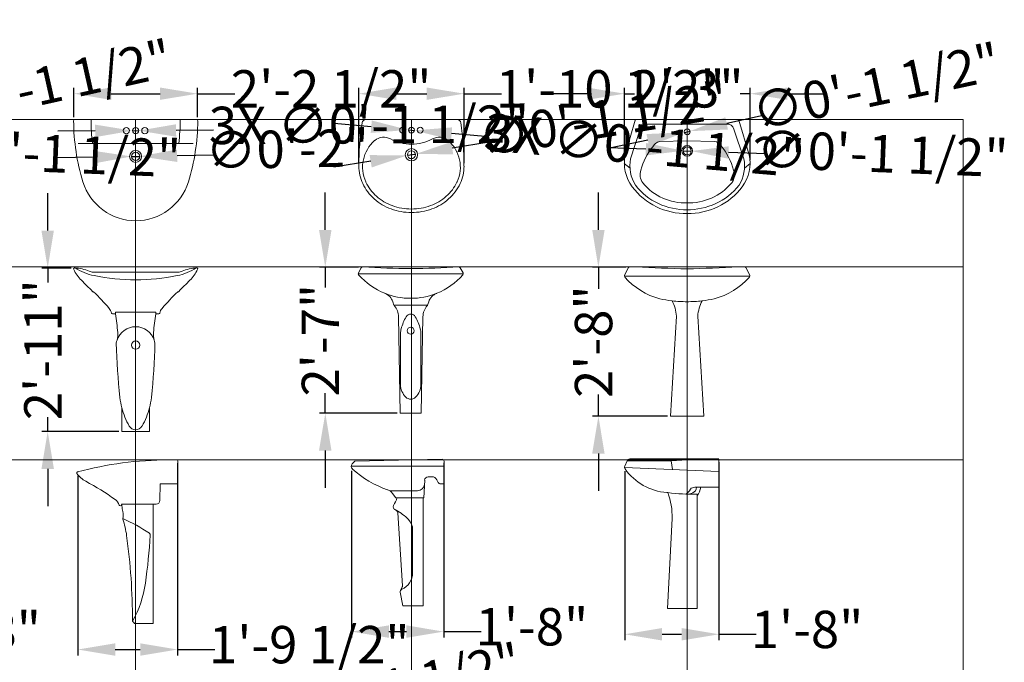
# Model space of a CAD drawing. Units: inches. Extents: x 2138 to 3265, y 2149 to 3392.
# Tile 13 of 13: x 3040 to 3251, y 3255 to 3392. Entities that reach past the tile are written whole.
import ezdxf

# ---------------------------------------------------------------- set-up
doc = ezdxf.new("R2010")
doc.units = ezdxf.units.IN
for name, color, linetype, lineweight in [('A-ANNO-DIMS', 2, 'Continuous', 18), ('A-DETL-GRID', 1, 'Continuous', 13), ('Washbasin-detail', 251, 'Continuous', 13), ('Washbasin-outline', 250, 'Continuous', 20)]:
    doc.layers.add(name, color=color, linetype=linetype, lineweight=lineweight)
doc.styles.get("Standard").update_dxf_attribs({"font": 'arial.ttf'})
doc.dimstyles.new('ISO-25', dxfattribs={"dimtxt": 8, "dimasz": 8, "dimexe": 1.25, "dimexo": 0.625, "dimtad": 0, "dimdec": 1, "dimlunit": 4, "dimtxsty": 'Standard', "dimcen": 2.5, "dimadec": 0, "dimazin": 0, "dimtfac": 1, "dimtdec": 1, "dimtmove": 0, "dimatfit": 3, "dimfxl": 1, "dimarcsym": 0})

# ---------------------------------------------------------------- blocks, each defined once
blk = doc.blocks.new('*D69')
at = {"layer": 'A-ANNO-DIMS', "color": 0, "lineweight": -2, "transparency": 16777216}
for p, q in [((2993.28, 3295.6), (2993.28, 3259.31)), ((3013.46, 3297.45), (3013.46, 3259.31)), ((3001.28, 3260.56), (3005.46, 3260.56)), ((3013.46, 3260.56), (3021.46, 3260.56))]:
    blk.add_line(p, q, dxfattribs=at)
at = {"layer": 'A-ANNO-DIMS', "color": 0, "transparency": 16777216}
for points in [[(3001.28, 3261.89), (3001.28, 3259.22), (2993.28, 3260.56)], [(3005.46, 3261.89), (3005.46, 3259.22), (3013.46, 3260.56)]]:
    blk.add_solid(points, dxfattribs=at)
at = {"layer": 'Defpoints', "color": 0, "transparency": 16777216}
for p in [(3013.46, 3298.07), (2993.28, 3296.23), (3013.46, 3260.56)]:
    blk.add_point(p, dxfattribs=at)
at = {"layer": 'A-ANNO-DIMS', "color": 0, "transparency": 16777216, "insert": (3032.34, 3260.56), "char_height": 8, "attachment_point": 5}
blk.add_mtext('1\'-8"', dxfattribs=at)
blk = doc.blocks.new('*D70')
at = {"layer": 'A-ANNO-DIMS', "color": 0, "lineweight": -2, "transparency": 16777216}
for p, q in [((3051.46, 3371.46), (3051.46, 3377.71)), ((3077.9, 3371.46), (3077.9, 3377.71)), ((3059.46, 3376.46), (3069.9, 3376.46)), ((3077.9, 3376.46), (3085.9, 3376.46))]:
    blk.add_line(p, q, dxfattribs=at)
at = {"layer": 'A-ANNO-DIMS', "color": 0, "transparency": 16777216}
for points in [[(3059.46, 3377.79), (3059.46, 3375.13), (3051.46, 3376.46)], [(3069.9, 3377.79), (3069.9, 3375.13), (3077.9, 3376.46)]]:
    blk.add_solid(points, dxfattribs=at)
at = {"layer": 'Defpoints', "color": 0, "transparency": 16777216}
for p in [(3077.9, 3376.46), (3051.46, 3370.84), (3077.9, 3370.84)]:
    blk.add_point(p, dxfattribs=at)
at = {"layer": 'A-ANNO-DIMS', "color": 0, "transparency": 16777216, "insert": (3106.55, 3376.46), "char_height": 8, "attachment_point": 5}
blk.add_mtext('2\'-2 1/2"', dxfattribs=at)
blk = doc.blocks.new('*D71')
at = {"layer": 'A-ANNO-DIMS', "color": 0, "lineweight": -2, "transparency": 16777216}
for p, q in [((3045.85, 3347.15), (3045.85, 3355.15)), ((3050.9, 3339.15), (3044.6, 3339.15)), ((3045.85, 3339.15), (3045.85, 3336.08)), ((3045.85, 3304.14), (3045.85, 3307.21)), ((3061.11, 3304.14), (3044.6, 3304.14)), ((3045.85, 3296.14), (3045.85, 3288.14))]:
    blk.add_line(p, q, dxfattribs=at)
at = {"layer": 'A-ANNO-DIMS', "color": 0, "transparency": 16777216}
for points in [[(3044.51, 3347.15), (3047.18, 3347.15), (3045.85, 3339.15)], [(3044.51, 3296.14), (3047.18, 3296.14), (3045.85, 3304.14)]]:
    blk.add_solid(points, dxfattribs=at)
at = {"layer": 'Defpoints', "color": 0, "transparency": 16777216}
for p in [(3051.53, 3339.15), (3045.85, 3304.14), (3061.73, 3304.14)]:
    blk.add_point(p, dxfattribs=at)
at = {"layer": 'A-ANNO-DIMS', "color": 0, "transparency": 16777216, "insert": (3045.85, 3321.65), "char_height": 8, "attachment_point": 5, "rotation": 90}
blk.add_mtext('2\'-11"', dxfattribs=at)
blk = doc.blocks.new('*D72')
at = {"layer": 'A-ANNO-DIMS', "color": 0, "lineweight": -2, "transparency": 16777216}
for p, q in [((3073.65, 3297.38), (3073.65, 3256.24)), ((3052.31, 3294.65), (3052.31, 3256.24)), ((3060.31, 3257.49), (3065.65, 3257.49)), ((3073.65, 3257.49), (3081.65, 3257.49))]:
    blk.add_line(p, q, dxfattribs=at)
at = {"layer": 'A-ANNO-DIMS', "color": 0, "transparency": 16777216}
for points in [[(3060.31, 3258.82), (3060.31, 3256.15), (3052.31, 3257.49)], [(3065.65, 3258.82), (3065.65, 3256.15), (3073.65, 3257.49)]]:
    blk.add_solid(points, dxfattribs=at)
at = {"layer": 'Defpoints', "color": 0, "transparency": 16777216}
for p in [(3073.65, 3298.01), (3052.31, 3295.28), (3073.65, 3257.49)]:
    blk.add_point(p, dxfattribs=at)
at = {"layer": 'A-ANNO-DIMS', "color": 0, "transparency": 16777216, "insert": (3101.86, 3257.49), "char_height": 8, "attachment_point": 5}
blk.add_mtext('1\'-9 1/2"', dxfattribs=at)
blk = doc.blocks.new('*D73')
at = {"layer": 'A-ANNO-DIMS', "color": 0, "lineweight": -2, "transparency": 16777216}
for p, q in [((3112.48, 3361.59), (3112.48, 3377.71)), ((3135, 3361.59), (3135, 3377.71)), ((3120.48, 3376.46), (3127, 3376.46)), ((3135, 3376.46), (3143, 3376.46))]:
    blk.add_line(p, q, dxfattribs=at)
at = {"layer": 'A-ANNO-DIMS', "color": 0, "transparency": 16777216}
for points in [[(3120.48, 3377.79), (3120.48, 3375.13), (3112.48, 3376.46)], [(3127, 3377.79), (3127, 3375.13), (3135, 3376.46)]]:
    blk.add_solid(points, dxfattribs=at)
at = {"layer": 'Defpoints', "color": 0, "transparency": 16777216}
for p in [(3135, 3376.46), (3112.48, 3360.96), (3135, 3360.96)]:
    blk.add_point(p, dxfattribs=at)
at = {"layer": 'A-ANNO-DIMS', "color": 0, "transparency": 16777216, "insert": (3166.31, 3376.46), "char_height": 8, "attachment_point": 5}
blk.add_mtext('1\'-10 1/2"', dxfattribs=at)
blk = doc.blocks.new('*D74')
at = {"layer": 'A-ANNO-DIMS', "color": 0, "lineweight": -2, "transparency": 16777216}
for p, q in [((3105.29, 3347.3), (3105.29, 3355.3)), ((3112.41, 3339.3), (3104.04, 3339.3)), ((3105.29, 3339.3), (3105.29, 3335.01)), ((3105.29, 3308.08), (3105.29, 3312.36)), ((3120.71, 3308.08), (3104.04, 3308.08)), ((3105.29, 3300.08), (3105.29, 3292.08))]:
    blk.add_line(p, q, dxfattribs=at)
at = {"layer": 'A-ANNO-DIMS', "color": 0, "transparency": 16777216}
for points in [[(3103.95, 3347.3), (3106.62, 3347.3), (3105.29, 3339.3)], [(3103.95, 3300.08), (3106.62, 3300.08), (3105.29, 3308.08)]]:
    blk.add_solid(points, dxfattribs=at)
at = {"layer": 'Defpoints', "color": 0, "transparency": 16777216}
for p in [(3113.03, 3339.3), (3105.29, 3308.08), (3121.34, 3308.08)]:
    blk.add_point(p, dxfattribs=at)
at = {"layer": 'A-ANNO-DIMS', "color": 0, "transparency": 16777216, "insert": (3105.29, 3323.69), "char_height": 8, "attachment_point": 5, "rotation": 90}
blk.add_mtext('2\'-7"', dxfattribs=at)
blk = doc.blocks.new('*D75')
at = {"layer": 'A-ANNO-DIMS', "color": 0, "lineweight": -2, "transparency": 16777216}
for p, q in [((3110.91, 3295.76), (3110.91, 3260.07)), ((3130.66, 3297.42), (3130.66, 3260.07)), ((3118.91, 3261.32), (3122.66, 3261.32)), ((3130.66, 3261.32), (3138.66, 3261.32))]:
    blk.add_line(p, q, dxfattribs=at)
at = {"layer": 'A-ANNO-DIMS', "color": 0, "transparency": 16777216}
for points in [[(3118.91, 3262.66), (3118.91, 3259.99), (3110.91, 3261.32)], [(3122.66, 3262.66), (3122.66, 3259.99), (3130.66, 3261.32)]]:
    blk.add_solid(points, dxfattribs=at)
at = {"layer": 'Defpoints', "color": 0, "transparency": 16777216}
for p in [(3130.66, 3298.04), (3110.91, 3296.39), (3130.66, 3261.32)]:
    blk.add_point(p, dxfattribs=at)
at = {"layer": 'A-ANNO-DIMS', "color": 0, "transparency": 16777216, "insert": (3149.54, 3261.32), "char_height": 8, "attachment_point": 5}
blk.add_mtext('1\'-8"', dxfattribs=at)
blk = doc.blocks.new('*D76')
at = {"layer": 'A-ANNO-DIMS', "color": 0, "lineweight": -2, "transparency": 16777216}
for p, q in [((3169.33, 3362.21), (3169.33, 3377.71)), ((3196.26, 3362.21), (3196.26, 3377.71)), ((3161.33, 3376.46), (3153.33, 3376.46)), ((3169.33, 3376.46), (3171.47, 3376.46)), ((3196.26, 3376.46), (3194.12, 3376.46)), ((3204.26, 3376.46), (3212.26, 3376.46))]:
    blk.add_line(p, q, dxfattribs=at)
at = {"layer": 'A-ANNO-DIMS', "color": 0, "transparency": 16777216}
for points in [[(3161.33, 3377.79), (3161.33, 3375.13), (3169.33, 3376.46)], [(3204.26, 3377.79), (3204.26, 3375.13), (3196.26, 3376.46)]]:
    blk.add_solid(points, dxfattribs=at)
at = {"layer": 'Defpoints', "color": 0, "transparency": 16777216}
for p in [(3196.26, 3376.46), (3169.33, 3361.58), (3196.26, 3361.58)]:
    blk.add_point(p, dxfattribs=at)
at = {"layer": 'A-ANNO-DIMS', "color": 0, "transparency": 16777216, "insert": (3182.8, 3376.46), "char_height": 8, "attachment_point": 5}
blk.add_mtext('2\'-3"', dxfattribs=at)
blk = doc.blocks.new('*D77')
at = {"layer": 'A-ANNO-DIMS', "color": 0, "lineweight": -2, "transparency": 16777216}
for p, q in [((3163.77, 3347.31), (3163.77, 3355.31)), ((3169.65, 3339.31), (3162.52, 3339.31)), ((3163.77, 3339.31), (3163.77, 3334.7)), ((3163.77, 3307.44), (3163.77, 3312.05)), ((3178.59, 3307.44), (3162.52, 3307.44)), ((3163.77, 3299.44), (3163.77, 3291.44))]:
    blk.add_line(p, q, dxfattribs=at)
at = {"layer": 'A-ANNO-DIMS', "color": 0, "transparency": 16777216}
for points in [[(3162.44, 3347.31), (3165.1, 3347.31), (3163.77, 3339.31)], [(3162.44, 3299.44), (3165.1, 3299.44), (3163.77, 3307.44)]]:
    blk.add_solid(points, dxfattribs=at)
at = {"layer": 'Defpoints', "color": 0, "transparency": 16777216}
for p in [(3170.27, 3339.31), (3163.77, 3307.44), (3179.21, 3307.44)]:
    blk.add_point(p, dxfattribs=at)
at = {"layer": 'A-ANNO-DIMS', "color": 0, "transparency": 16777216, "insert": (3163.77, 3323.38), "char_height": 8, "attachment_point": 5, "rotation": 90}
blk.add_mtext('2\'-8"', dxfattribs=at)
blk = doc.blocks.new('*D78')
at = {"layer": 'A-ANNO-DIMS', "color": 0, "lineweight": -2, "transparency": 16777216}
for p, q in [((3189.57, 3297.61), (3189.57, 3259.5)), ((3169.41, 3295.65), (3169.41, 3259.5)), ((3177.41, 3260.75), (3181.57, 3260.75)), ((3189.57, 3260.75), (3197.57, 3260.75))]:
    blk.add_line(p, q, dxfattribs=at)
at = {"layer": 'A-ANNO-DIMS', "color": 0, "transparency": 16777216}
for points in [[(3177.41, 3262.09), (3177.41, 3259.42), (3169.41, 3260.75)], [(3181.57, 3262.09), (3181.57, 3259.42), (3189.57, 3260.75)]]:
    blk.add_solid(points, dxfattribs=at)
at = {"layer": 'Defpoints', "color": 0, "transparency": 16777216}
for p in [(3189.57, 3298.23), (3169.41, 3296.27), (3189.57, 3260.75)]:
    blk.add_point(p, dxfattribs=at)
at = {"layer": 'A-ANNO-DIMS', "color": 0, "transparency": 16777216, "insert": (3208.45, 3260.75), "char_height": 8, "attachment_point": 5}
blk.add_mtext('1\'-8"', dxfattribs=at)
blk = doc.blocks.new('*D113')
at = {"layer": 'A-ANNO-DIMS', "color": 0, "lineweight": -2, "transparency": 16777216}
for p, q in [((3021.86, 3371.95), (3014.05, 3370.2)), ((3005.01, 3368.17), (3006.24, 3368.45)), ((2997.21, 3366.42), (2989.4, 3364.68))]:
    blk.add_line(p, q, dxfattribs=at)
at = {"layer": 'A-ANNO-DIMS', "color": 0, "transparency": 16777216}
for points in [[(3013.76, 3371.5), (3014.34, 3368.9), (3006.24, 3368.45)], [(2996.92, 3367.73), (2997.5, 3365.12), (3005.01, 3368.17)]]:
    blk.add_solid(points, dxfattribs=at)
at = {"layer": 'Defpoints', "color": 0, "transparency": 16777216}
for p in [(3005.01, 3368.17), (3006.24, 3368.45)]:
    blk.add_point(p, dxfattribs=at)
at = {"layer": 'A-ANNO-DIMS', "color": 0, "transparency": 16777216, "insert": (3046.18, 3377.39), "char_height": 8, "attachment_point": 5, "rotation": 12.6253}
blk.add_mtext('∅0\'-1 1/2"', dxfattribs=at)
blk = doc.blocks.new('*D114')
at = {"layer": 'A-ANNO-DIMS', "color": 0, "lineweight": -2, "transparency": 16777216}
for p, q in [((2996.77, 3364.56), (2988.77, 3364.88)), ((3004.76, 3364.25), (3006.49, 3364.18)), ((3022.48, 3363.55), (3014.49, 3363.87))]:
    blk.add_line(p, q, dxfattribs=at)
at = {"layer": 'A-ANNO-DIMS', "color": 0, "transparency": 16777216}
for points in [[(2996.82, 3365.9), (2996.72, 3363.23), (3004.76, 3364.25)], [(3014.54, 3365.2), (3014.44, 3362.54), (3006.49, 3364.18)]]:
    blk.add_solid(points, dxfattribs=at)
at = {"layer": 'Defpoints', "color": 0, "transparency": 16777216}
for p in [(3004.76, 3364.25), (3006.49, 3364.18)]:
    blk.add_point(p, dxfattribs=at)
at = {"layer": 'A-ANNO-DIMS', "color": 0, "transparency": 16777216, "insert": (3047.39, 3362.58), "char_height": 8, "attachment_point": 5, "rotation": 357.7522}
blk.add_mtext('∅0\'-1 1/2"', dxfattribs=at)
blk = doc.blocks.new('*D115')
at = {"layer": 'A-ANNO-DIMS', "color": 0, "lineweight": -2, "transparency": 16777216}
for p, q in [((3056.01, 3368.51), (3048.01, 3368.47)), ((3064.01, 3368.54), (3065.35, 3368.55)), ((3081.35, 3368.62), (3073.35, 3368.59))]:
    blk.add_line(p, q, dxfattribs=at)
at = {"layer": 'A-ANNO-DIMS', "color": 0, "transparency": 16777216}
for points in [[(3056.01, 3369.84), (3056.02, 3367.17), (3064.01, 3368.54)], [(3073.35, 3369.92), (3073.36, 3367.25), (3065.35, 3368.55)]]:
    blk.add_solid(points, dxfattribs=at)
at = {"layer": 'Defpoints', "color": 0, "transparency": 16777216}
for p in [(3064.01, 3368.54), (3065.35, 3368.55)]:
    blk.add_point(p, dxfattribs=at)
at = {"layer": 'A-ANNO-DIMS', "color": 0, "transparency": 16777216, "insert": (3114.66, 3368.78), "char_height": 8, "attachment_point": 5, "rotation": 0.2663}
blk.add_mtext('3X ∅0\'-1 1/2"', dxfattribs=at)
blk = doc.blocks.new('*D116')
at = {"layer": 'A-ANNO-DIMS', "color": 0, "lineweight": -2, "transparency": 16777216}
for p, q in [((3055.8, 3362.89), (3047.8, 3362.75)), ((3063.8, 3363.02), (3065.57, 3363.05)), ((3081.57, 3363.32), (3073.57, 3363.18))]:
    blk.add_line(p, q, dxfattribs=at)
at = {"layer": 'A-ANNO-DIMS', "color": 0, "transparency": 16777216}
for points in [[(3055.78, 3364.22), (3055.82, 3361.55), (3063.8, 3363.02)], [(3073.55, 3364.52), (3073.59, 3361.85), (3065.57, 3363.05)]]:
    blk.add_solid(points, dxfattribs=at)
at = {"layer": 'Defpoints', "color": 0, "transparency": 16777216}
for p in [(3063.8, 3363.02), (3065.57, 3363.05)]:
    blk.add_point(p, dxfattribs=at)
at = {"layer": 'A-ANNO-DIMS', "color": 0, "transparency": 16777216, "insert": (3097.17, 3363.58), "char_height": 8, "attachment_point": 5, "rotation": 0.9632}
blk.add_mtext('∅0\'-2"', dxfattribs=at)
blk = doc.blocks.new('*D117')
at = {"layer": 'A-ANNO-DIMS', "color": 0, "lineweight": -2, "transparency": 16777216}
for p, q in [((3115.13, 3369.4), (3107.16, 3370.08)), ((3123.1, 3368.71), (3124.37, 3368.6)), ((3140.32, 3367.24), (3132.34, 3367.92))]:
    blk.add_line(p, q, dxfattribs=at)
at = {"layer": 'A-ANNO-DIMS', "color": 0, "transparency": 16777216}
for points in [[(3115.25, 3370.72), (3115.02, 3368.07), (3123.1, 3368.71)], [(3132.46, 3369.25), (3132.23, 3366.59), (3124.37, 3368.6)]]:
    blk.add_solid(points, dxfattribs=at)
at = {"layer": 'Defpoints', "color": 0, "transparency": 16777216}
for p in [(3123.1, 3368.71), (3124.37, 3368.6)]:
    blk.add_point(p, dxfattribs=at)
at = {"layer": 'A-ANNO-DIMS', "color": 0, "transparency": 16777216, "insert": (3173.5, 3364.39), "char_height": 8, "attachment_point": 5, "rotation": 355.1005}
blk.add_mtext('3X ∅0\'-1 1/2"', dxfattribs=at)
blk = doc.blocks.new('*D118')
at = {"layer": 'A-ANNO-DIMS', "color": 0, "lineweight": -2, "transparency": 16777216}
for p, q in [((3140.37, 3366.1), (3132.47, 3364.82)), ((3122.9, 3363.27), (3124.57, 3363.54)), ((3115.01, 3361.99), (3107.11, 3360.71))]:
    blk.add_line(p, q, dxfattribs=at)
at = {"layer": 'A-ANNO-DIMS', "color": 0, "transparency": 16777216}
for points in [[(3132.26, 3366.13), (3132.68, 3363.5), (3124.57, 3363.54)], [(3114.79, 3363.31), (3115.22, 3360.67), (3122.9, 3363.27)]]:
    blk.add_solid(points, dxfattribs=at)
at = {"layer": 'Defpoints', "color": 0, "transparency": 16777216}
for p in [(3122.9, 3363.27), (3124.57, 3363.54)]:
    blk.add_point(p, dxfattribs=at)
at = {"layer": 'A-ANNO-DIMS', "color": 0, "transparency": 16777216, "insert": (3164.98, 3370.08), "char_height": 8, "attachment_point": 5, "rotation": 9.1943}
blk.add_mtext('∅0\'-1 1/2"', dxfattribs=at)
blk = doc.blocks.new('*D119')
at = {"layer": 'A-ANNO-DIMS', "color": 0, "lineweight": -2, "transparency": 16777216}
for p, q in [((3199.06, 3371.76), (3191.24, 3370.1)), ((3182.18, 3368.18), (3183.41, 3368.44)), ((3174.35, 3366.52), (3166.53, 3364.86))]:
    blk.add_line(p, q, dxfattribs=at)
at = {"layer": 'A-ANNO-DIMS', "color": 0, "transparency": 16777216}
for points in [[(3190.96, 3371.41), (3191.51, 3368.8), (3183.41, 3368.44)], [(3174.07, 3367.82), (3174.63, 3365.22), (3182.18, 3368.18)]]:
    blk.add_solid(points, dxfattribs=at)
at = {"layer": 'Defpoints', "color": 0, "transparency": 16777216}
for p in [(3182.18, 3368.18), (3183.41, 3368.44)]:
    blk.add_point(p, dxfattribs=at)
at = {"layer": 'A-ANNO-DIMS', "color": 0, "transparency": 16777216, "insert": (3223.45, 3376.94), "char_height": 8, "attachment_point": 5, "rotation": 11.979}
blk.add_mtext('∅0\'-1 1/2"', dxfattribs=at)
blk = doc.blocks.new('*D120')
at = {"layer": 'A-ANNO-DIMS', "color": 0, "lineweight": -2, "transparency": 16777216}
for p, q in [((3173.93, 3364.56), (3165.94, 3364.87)), ((3181.93, 3364.25), (3183.66, 3364.18)), ((3199.65, 3363.56), (3191.65, 3363.87))]:
    blk.add_line(p, q, dxfattribs=at)
at = {"layer": 'A-ANNO-DIMS', "color": 0, "transparency": 16777216}
for points in [[(3173.99, 3365.89), (3173.88, 3363.23), (3181.93, 3364.25)], [(3191.7, 3365.2), (3191.6, 3362.54), (3183.66, 3364.18)]]:
    blk.add_solid(points, dxfattribs=at)
at = {"layer": 'Defpoints', "color": 0, "transparency": 16777216}
for p in [(3181.93, 3364.25), (3183.66, 3364.18)]:
    blk.add_point(p, dxfattribs=at)
at = {"layer": 'A-ANNO-DIMS', "color": 0, "transparency": 16777216, "insert": (3224.56, 3362.59), "char_height": 8, "attachment_point": 5, "rotation": 357.7634}
blk.add_mtext('∅0\'-1 1/2"', dxfattribs=at)
blk = doc.blocks.new('*D125')
at = {"layer": 'A-ANNO-DIMS', "color": 0, "lineweight": -2, "transparency": 16777216}
for p, q in [((3080.99, 3240.1), (3073.17, 3238.45)), ((3064.03, 3236.52), (3065.34, 3236.8)), ((3056.2, 3234.87), (3048.37, 3233.21))]:
    blk.add_line(p, q, dxfattribs=at)
at = {"layer": 'A-ANNO-DIMS', "color": 0, "transparency": 16777216}
for points in [[(3072.89, 3239.75), (3073.44, 3237.14), (3065.34, 3236.8)], [(3055.93, 3236.17), (3056.48, 3233.56), (3064.03, 3236.52)]]:
    blk.add_solid(points, dxfattribs=at)
at = {"layer": 'Defpoints', "color": 0, "transparency": 16777216}
for p in [(3064.03, 3236.52), (3065.34, 3236.8)]:
    blk.add_point(p, dxfattribs=at)
at = {"layer": 'A-ANNO-DIMS', "color": 0, "transparency": 16777216, "insert": (3113.58, 3246.98), "char_height": 8, "attachment_point": 5, "rotation": 11.9181}
blk.add_mtext('3X ∅0\'-1 1/2"', dxfattribs=at)

msp = doc.modelspace()

# ---------------------------------------------------------------- linework, layer by layer
at = {"layer": 'A-DETL-GRID'}
for p, q in [((2828.46, 3370.91), (3241.85, 3370.91)), ((3064.68, 3239.02), (3064.68, 3370.91)), ((3123.74, 3239.02), (3123.74, 3370.91)), ((3182.79, 3239.02), (3182.79, 3370.91)), ((3241.85, 3239.02), (3241.85, 3370.91)), ((2828.46, 3339.41), (3241.85, 3339.41)), ((2828.46, 3298.07), (3241.85, 3298.07))]:
    msp.add_line(p, q, dxfattribs=at)
at = {"layer": 'Washbasin-detail'}
for p, q in [((3170.54, 3360.51), (3169.32, 3361.5)), ((3195.05, 3360.51), (3196.27, 3361.5)), ((3064.68, 3338.27), (3055.63, 3338.27)), ((3064.68, 3338.27), (3073.74, 3338.27)), ((3112.33, 3337.91), (3123.59, 3337.91)), ((3113.31, 3339.41), (3123.59, 3339.41)), ((3133.87, 3339.41), (3123.59, 3339.41)), ((3134.84, 3337.91), (3123.59, 3337.91)), ((3120.03, 3331.16), (3123.59, 3331.16)), ((3127.15, 3331.16), (3123.59, 3331.16)), ((3121.4, 3325.14), (3121.4, 3314.2)), ((3125.77, 3325.14), (3125.77, 3314.2)), ((3061.73, 3304.14), (3061.73, 3309.2)), ((3067.64, 3304.14), (3067.64, 3309.2)), ((3064.68, 3304.14), (3061.73, 3304.14)), ((3064.68, 3304.14), (3067.64, 3304.14)), ((3110.84, 3296.71), (3130.72, 3296.71)), ((3120.63, 3289.95), (3126.24, 3289.95)), ((3061.8, 3288.63), (3068.41, 3288.63)), ((3061.8, 3288.63), (3062.61, 3288.63)), ((3123.99, 3283.2), (3123.99, 3273.86))]:
    msp.add_line(p, q, dxfattribs=at)
for points in [[(3182.79, 3369.92), (3174.29, 3369.92, 0.390337), (3172.71, 3368.9), (3170.66, 3362.55, 0.183446), (3171.69, 3356.85, 0.232242), (3182.79, 3351.62, 0.646667)], [(3182.79, 3369.92), (3191.19, 3369.92, -0.390337), (3192.76, 3368.9), (3194.94, 3362.55, -0.183446), (3193.9, 3356.85, -0.230237), (3182.68, 3351.62, -0.646667)], [(3113.96, 3357.61, 0.00234), (3113.99, 3357.54, 0.102555), (3116.27, 3354.5, 0.093464), (3119.63, 3352.5, 0.087915), (3123.74, 3351.77, 0.087915)], [(3133.51, 3357.61, -0.00234), (3133.48, 3357.54, -0.102555), (3131.2, 3354.5, -0.093464), (3127.85, 3352.5, -0.087915), (3123.74, 3351.77, -0.087915)], [(3182.79, 3338.98, -0.010807), (3171.81, 3339.41, -32.766404)], [(3182.74, 3338.98, 0.010807), (3193.73, 3339.41, 32.766404)], [(3184.76, 3292.21, -0.342017), (3183.97, 3291.03, -0.117748), (3182.71, 3290.71, 189.338615)], [(3185.67, 3292.21, -0.172288), (3184.92, 3290.45, 0.079687)]]:
    msp.add_lwpolyline(points, format="xyb", dxfattribs=at)
for points in [[(3182.79, 3337.41), (3169.37, 3337.41)], [(3182.74, 3337.41), (3196.17, 3337.41)], [(3169.92, 3297.88), (3179.37, 3297.88), (3186.22, 3298.27)], [(3179.37, 3297.88), (3179.64, 3296)], [(3169.37, 3296.42), (3189.57, 3295.59)]]:
    msp.add_lwpolyline(points, dxfattribs=at)
for centre, radius in [((3062.71, 3368.55), 0.669), ((3064.68, 3368.55), 0.669), ((3066.65, 3368.55), 0.669), ((3121.86, 3368.66), 0.638), ((3125.61, 3368.66), 0.638), ((3182.79, 3368.31), 0.63), ((3182.79, 3364.22), 1.14), ((3182.79, 3364.22), 0.866), ((3064.68, 3363.04), 1.28), ((3064.68, 3363.04), 0.886), ((3123.74, 3363.4), 1.31), ((3123.59, 3325.72), 0.751), ((3064.68, 3322.64), 0.886)]:
    msp.add_circle(centre, radius, dxfattribs=at)
for centre, radius, start, end in [((3096.66, 3370.9), 41.53, 179.9856, 187.0649), ((3032.7, 3370.9), 41.53, 352.9351, 0.0144), ((3123.74, 3368.66), 0.638, 90, 270), ((3123.74, 3368.66), 0.638, 270, 90), ((3117.83, 3364.15), 3, 61.4965, 130.9137), ((3129.65, 3364.15), 3, 49.0863, 118.5035), ((3120.78, 3360.75), 7.51, 130.9137, 204.754), ((3123.74, 3375.04), 9.38, 241.4965, 270), ((3123.74, 3375.04), 9.38, 270, 298.5035), ((3126.7, 3360.75), 7.51, 335.246, 49.0863), ((3123.74, 3363.4), 0.844, 90, 270), ((3123.74, 3363.4), 0.844, 270, 90), ((3050.96, 3329.36), 9.84, 67.5001, 85.9904), ((3055.63, 3340.64), 2.36, 247.5001, 270), ((3073.74, 3340.64), 2.36, 270, 292.4999), ((3078.41, 3329.36), 9.84, 94.0096, 112.4999), ((3123.59, 3328.16), 1.13, 90, 150.274), ((3123.59, 3328.16), 1.13, 29.726, 90), ((3132.39, 3323.13), 11.26, 150.274, 164.5121), ((3114.79, 3323.13), 11.26, 15.4879, 29.726), ((3125.15, 3325.14), 3.75, 164.5121, 180), ((3122.02, 3325.14), 3.75, 0, 15.4879), ((3125.15, 3314.2), 3.75, 180, 225.9297), ((3122.02, 3314.2), 3.75, 314.0703, 0), ((3123.59, 3312.58), 1.5, 225.9297, 270), ((3123.59, 3312.58), 1.5, 270, 314.0703), ((3115.12, 3277.39), 11.26, 44.6785, 61.8252), ((3049.56, 3256.55), 31.5, 55.0237, 66.9079), ((3120.99, 3283.2), 3, 0, 44.6785), ((2934.23, 3290.44), 133.86, 351.9594, 356.3821), ((3067.43, 3282.01), 0.394, 356.3821, 61.0641), ((3120.24, 3273.86), 3.75, 292.458, 0), ((3043.38, 3275.02), 23.62, 330.9388, 351.9594)]:
    msp.add_arc(centre, radius, start, end, dxfattribs=at)
at = {"layer": 'Washbasin-outline'}
for p, q in [((3051.63, 3370.91), (3077.73, 3370.91)), ((3113.93, 3370.91), (3123.74, 3370.91)), ((3133.55, 3370.91), (3123.74, 3370.91)), ((3052.35, 3365.79), (3064.68, 3365.79)), ((3077.02, 3365.79), (3064.68, 3365.79)), ((3112.97, 3339.21), (3112.37, 3338.09)), ((3134.2, 3339.21), (3134.8, 3338.09)), ((3169.36, 3337.59), (3170.22, 3339.24)), ((3170.51, 3339.41), (3182.79, 3339.41)), ((3195.02, 3339.41), (3182.74, 3339.41)), ((3196.18, 3337.59), (3195.31, 3339.24)), ((3055.68, 3334.06), (3055.59, 3334.06)), ((3073.69, 3334.06), (3073.78, 3334.06)), ((3120, 3331.21), (3119.75, 3331.94)), ((3127.15, 3331.16), (3127.43, 3331.94)), ((3060.36, 3329.34), (3059.74, 3329.34)), ((3060.36, 3329.34), (3060.36, 3329.73)), ((3064.68, 3329.73), (3060.36, 3329.73)), ((3064.68, 3329.73), (3069.01, 3329.73)), ((3069.01, 3329.34), (3069.01, 3329.73)), ((3069.62, 3329.34), (3069.01, 3329.34)), ((3121.34, 3308.08), (3120.98, 3328.71)), ((3125.84, 3308.08), (3126.2, 3328.71)), ((3121.34, 3308.08), (3125.84, 3308.08)), ((3071.67, 3298.07), (3073.49, 3298.07)), ((3073.72, 3297.84), (3073.72, 3292.96)), ((3111.59, 3297.83), (3111.03, 3297.21)), ((3111.59, 3297.83), (3130.34, 3298.21)), ((3130.72, 3297.83), (3130.72, 3293.1)), ((3169.42, 3296.74), (3169.91, 3297.89)), ((3170.49, 3298.27), (3189.57, 3298.27)), ((3126.41, 3289.95), (3126.57, 3293.73)), ((3127.32, 3294.45), (3128.15, 3294.45)), ((3129.44, 3293.26), (3129.16, 3293.83)), ((3069.88, 3289.4), (3069.92, 3292.96)), ((3069.92, 3292.96), (3073.72, 3292.96)), ((3119.09, 3291.45), (3125.03, 3291.45)), ((3129.95, 3292.95), (3130.57, 3292.95)), ((3120.4, 3289.95), (3119.7, 3290.89)), ((3120.4, 3289.95), (3120.63, 3289.95)), ((3126.24, 3289.95), (3126.24, 3266.87)), ((3126.24, 3289.95), (3126.41, 3289.95)), ((3184.92, 3290.45), (3184.92, 3290.71)), ((3184.92, 3266.3), (3184.92, 3290.45)), ((3061.65, 3288.42), (3061.69, 3288.54)), ((3061.72, 3288.63), (3061.72, 3288.23)), ((3061.72, 3288.63), (3061.8, 3288.63)), ((3068.41, 3288.63), (3068.41, 3263.04)), ((3068.41, 3288.63), (3069.09, 3288.63)), ((3120.83, 3286.71), (3121.81, 3271.09)), ((3121.38, 3270.12), (3121.78, 3270.92)), ((3121.34, 3269.77), (3121.89, 3266.87)), ((3121.89, 3266.87), (3126.24, 3266.87)), ((3064.47, 3263.04), (3068.41, 3263.04))]:
    msp.add_line(p, q, dxfattribs=at)
for points in [[(3051.4, 3370.67, 0.07343), (3053.39, 3357.6, 0.07343)], [(3182.79, 3370.91), (3171.81, 3370.91, 0.349334), (3171.62, 3370.76), (3169.5, 3363.39, 0.210862), (3171.01, 3356.53, 0.238221), (3182.75, 3350.79, -0.006376)], [(3182.79, 3370.91), (3193.67, 3370.91, -0.349334), (3193.86, 3370.76), (3196.09, 3363.39, -0.210862), (3194.58, 3356.53, -0.236938), (3182.76, 3350.79, 0.006376)], [(3182.79, 3366.34), (3176.83, 3366.24, 0.204561), (3175.43, 3365.12, 0.107345), (3172.89, 3360.11, 0.24654), (3173.27, 3357.37, 0.234802), (3182.83, 3353.11, 0.791678)], [(3182.68, 3366.34), (3188.64, 3366.24, -0.218686), (3190.04, 3365.32, -0.103144), (3192.71, 3360.11, -0.24654), (3192.33, 3357.37, -0.232404), (3182.64, 3353.11, -0.791678)], [(3112.48, 3360.96, 0.11006), (3113.31, 3357.22, 0.102555), (3115.78, 3353.93, 0.093464), (3119.37, 3351.8, 0.087915), (3123.74, 3351.02, 0.087915)], [(3135, 3360.96, -0.11006), (3134.16, 3357.22, -0.102555), (3131.7, 3353.93, -0.093464), (3128.11, 3351.8, -0.087915), (3123.74, 3351.02, -0.087915)], [(3053.39, 3357.6, 0.329453), (3064.68, 3349.26, 0.329453), (3075.97, 3357.6, 0.329453)], [(3182.79, 3307.44), (3179.21, 3307.44), (3180.5, 3328.86, 0.094609), (3179.54, 3332.13, -1.525098)], [(3182.74, 3307.44), (3186.32, 3307.44), (3185.03, 3328.86, -0.094609), (3186, 3332.13, 1.525098)], [(3189.57, 3298.23), (3189.57, 3292.21), (3185.67, 3292.21, 0.240306)], [(3185.67, 3292.21), (3184.41, 3292.21, 0.240306), (3183.46, 3291.81, -0.219906), (3182.32, 3290.75, 6.2607)], [(3184.92, 3266.3), (3178.54, 3266.3), (3179.55, 3285.55, 0.103398), (3178.61, 3291.08, 5.161723)]]:
    msp.add_lwpolyline(points, format="xyb", dxfattribs=at)
for centre, radius, start, end in [((3051.63, 3370.67), 0.236, 90, 180.2872), ((3032.7, 3370.9), 45.28, 342.9141, 359.7128), ((3077.73, 3370.67), 0.236, 359.7128, 90), ((3174.46, 3360.96), 61.98, 171.3647, 180), ((3113.93, 3370.16), 0.751, 90, 171.3647), ((3133.55, 3370.16), 0.751, 4.4701, 90), ((3073.01, 3360.96), 61.98, 360, 8.6353), ((3051.63, 3338.94), 0.236, 85.9904, 205.7315), ((3059.22, 3342.6), 8.66, 205.7315, 224.658), ((3058.12, 3349.09), 11.81, 237.0913, 258.5261), ((3071.24, 3349.09), 11.81, 281.4739, 302.9087), ((3070.14, 3342.6), 8.66, 315.342, 334.2685), ((3077.73, 3338.94), 0.236, 334.2685, 94.0096), ((3112.7, 3337.91), 0.375, 151.9275, 221.7089), ((3123.59, 3347.61), 14.95, 221.7089, 248.1891), ((3113.31, 3339.04), 0.375, 90, 151.9275), ((3123.59, 3480.09), 141.05, 265.8197, 274.1803), ((3123.59, 3347.61), 14.95, 291.8109, 318.2911), ((3133.87, 3339.04), 0.375, 28.0725, 90), ((3134.47, 3337.91), 0.375, 318.2911, 28.0725), ((3169.65, 3337.44), 0.325, 152.4267, 221.363), ((3170.51, 3339.09), 0.325, 90, 152.4267), ((3195.02, 3339.09), 0.325, 27.5733, 90), ((3195.89, 3337.44), 0.325, 318.637, 27.5733), ((3012.28, 3293.8), 59.06, 43.0851, 46.3304), ((3064.68, 3381.41), 44.79, 258.5261, 270), ((3064.68, 3381.41), 44.79, 270, 281.4739), ((3117.08, 3293.8), 59.06, 133.6696, 136.9149), ((3180.87, 3347.32), 15.28, 221.363, 255.1139), ((3184.66, 3347.32), 15.28, 284.8861, 318.637), ((3055.59, 3334.3), 0.236, 223.0851, 270), ((3014.29, 3291.94), 59.06, 40.7487, 45.4966), ((3115.08, 3291.94), 59.06, 134.5034, 139.2513), ((3073.78, 3334.3), 0.236, 270, 316.9149), ((3123.59, 3347.61), 14.95, 248.1891, 270), ((3116.92, 3330.94), 3, 19.3487, 68.1891), ((3123.59, 3347.61), 14.95, 270, 291.8109), ((3130.26, 3330.94), 3, 111.8109, 160.6513), ((3126.82, 3331.33), 0.375, 319.3997, 340.6513), ((3182.97, 3361.5), 29.57, 258.2458, 263.3339), ((3182.97, 3361.5), 29.57, 258.2458, 263.3339), ((3182.97, 3361.5), 29.57, 263.3339, 269.6059), ((3182.56, 3361.5), 29.57, 270.3941, 276.6661), ((3182.56, 3361.5), 29.57, 276.6661, 281.7542), ((3057.23, 3328.95), 2.36, 13.5711, 40.7487), ((3059.74, 3329.55), 0.217, 193.5711, 270), ((2927.87, 3310.21), 133.86, 6.4962, 8.214), ((3201.49, 3310.21), 133.86, 171.786, 173.5038), ((3069.62, 3329.55), 0.217, 270, 346.4289), ((3072.13, 3328.95), 2.36, 139.2513, 166.4289), ((3117.22, 3328.65), 3.75, 0.9972, 40.6003), ((3129.95, 3328.65), 3.75, 139.3997, 179.0028), ((3064.68, 3322.39), 4.19, 90, 161.9506), ((3056.96, 3324.91), 3.94, 341.9506, 6.4962), ((3064.68, 3322.39), 4.19, 18.0494, 90), ((3072.41, 3324.91), 3.94, 173.5038, 198.0494), ((3064.68, 3322.39), 4.19, 161.9506, 170.6282), ((3060.79, 3323.04), 0.236, 170.6282, 181.2912), ((3194.37, 3326.05), 133.86, 181.2912, 186.2554), ((2934.99, 3326.05), 133.86, 353.7446, 358.7088), ((3064.68, 3322.39), 4.19, 9.3718, 18.0494), ((3068.58, 3323.04), 0.236, 358.7088, 9.3718), ((3076.97, 3313.18), 15.75, 186.2554, 194.6475), ((3052.4, 3313.18), 15.75, 345.3525, 353.7446), ((3076.97, 3313.18), 15.75, 194.6475, 209.9264), ((3052.4, 3313.18), 15.75, 330.0736, 345.3525), ((3064.68, 3306.11), 1.57, 209.9264, 270), ((3064.68, 3306.11), 1.57, 270, 330.0736), ((3071.67, 3223.27), 74.8, 90, 105.0541), ((3073.49, 3297.84), 0.236, 0, 90), ((3130.35, 3297.83), 0.375, 0, 91.146), ((3170.49, 3297.64), 0.63, 90, 156.9487), ((3052.31, 3295.28), 0.236, 80.1189, 216.9988), ((3111.59, 3296.71), 0.751, 138.1897, 228.0901), ((3126.12, 3312.9), 22.52, 228.0901, 250.5973), ((3170, 3296.49), 0.63, 156.9487, 215.1468), ((3179.22, 3302.98), 11.9, 215.1468, 266.1673), ((3056.83, 3298.69), 5.91, 216.9988, 241.6156), ((3025.95, 3241.54), 59.06, 54.4564, 61.6156), ((3127.32, 3293.7), 0.751, 90, 177.6141), ((3128.15, 3293.33), 1.13, 26.5651, 90), ((3129.95, 3293.52), 0.563, 206.5651, 270), ((3117.9, 3289.54), 2.25, 36.8699, 70.5973), ((3125.03, 3292.95), 1.5, 270, 357.6141), ((3130.57, 3293.1), 0.15, 270, 0), ((3058.91, 3287.67), 2.36, 18.3283, 54.4564), ((3069.09, 3289.41), 0.787, 270, 359.2881), ((3116.94, 3290.66), 3.75, 321.8003, 349.1251), ((3184.2, 3332.57), 41.86, 262.0734, 262.3523), ((3184.2, 3332.57), 41.86, 262.3523, 270.9902), ((3061.4, 3288.5), 0.263, 198.3283, 343.3008), ((3061.8, 3288.51), 0.118, 90, 163.3008), ((2930.14, 3263.61), 133.86, 10.0667, 10.5985), ((3058.06, 3286.32), 3.94, 348.3091, 10.0667), ((3120.59, 3288.07), 0.751, 159.4327, 250.0922), ((3115.12, 3277.39), 11.26, 61.8252, 62.3972), ((3120.08, 3286.65), 0.751, 3.6095, 61.8252), ((3062.15, 3285.48), 0.236, 168.3091, 198.413), ((3043.25, 3279.18), 19.69, 7.8387, 18.413), ((2930.14, 3263.61), 133.86, 359.9895, 7.8387), ((3121.89, 3269.87), 0.563, 112.458, 190.8069), ((3121.44, 3271.09), 0.375, 333.7188, 0.9972), ((3064.24, 3263.59), 0.236, 179.9895, 243.0336), ((3063.77, 3262.68), 0.787, 27.208, 63.0336)]:
    msp.add_arc(centre, radius, start, end, dxfattribs=at)

# ---------------------------------------------------------------- dimensions: what is measured, and where the dimension line sits
at = {"layer": 'A-ANNO-DIMS'}
for p1, p2, picture, middle in [((3005.01, 3368.17), (3006.24, 3368.45), '*D113', (3046.18, 3377.39)), ((3182.18, 3368.18), (3183.41, 3368.44), '*D119', (3223.45, 3376.94)), ((3122.9, 3363.27), (3124.57, 3363.54), '*D118', (3164.98, 3370.08)), ((3004.76, 3364.25), (3006.49, 3364.18), '*D114', (3047.39, 3362.58)), ((3181.93, 3364.25), (3183.66, 3364.18), '*D120', (3224.56, 3362.59)), ((3063.8, 3363.02), (3065.57, 3363.05), '*D116', (3097.17, 3363.58))]:
    dim = msp.add_diameter_dim_2p(p1=p1, p2=p2, dimstyle='ISO-25', override={"dimdec": 1, "dimlfac": 1, "dimrnd": 0, "dimzin": 1, "dimdsep": 46, "dimlunit": 4, "dimfrac": 2}, dxfattribs=at)
    dim.commit()
    dim.dimension.update_dxf_attribs({"geometry": picture, "text_midpoint": middle})
for base, p1, p2, picture, middle in [((3077.9, 3376.46), (3051.46, 3370.84), (3077.9, 3370.84), '*D70', (3106.55, 3376.46)), ((3135, 3376.46), (3112.48, 3360.96), (3135, 3360.96), '*D73', (3166.31, 3376.46)), ((3196.26, 3376.46), (3169.33, 3361.58), (3196.26, 3361.58), '*D76', (3182.8, 3376.46)), ((3013.46, 3260.56), (2993.28, 3296.23), (3013.46, 3298.07), '*D69', (3032.34, 3260.56)), ((3073.65, 3257.49), (3052.31, 3295.28), (3073.65, 3298.01), '*D72', (3101.86, 3257.49)), ((3130.6589, 3261.323), (3110.9065, 3296.3858), (3130.6589, 3298.0419), '*D75', (3149.5404, 3261.323)), ((3189.57, 3260.75), (3169.41, 3296.27), (3189.57, 3298.23), '*D78', (3208.45, 3260.75))]:
    dim = msp.add_linear_dim(base=base, p1=p1, p2=p2, dimstyle='ISO-25', override={"dimdec": 1, "dimlfac": 1, "dimrnd": 0, "dimzin": 1, "dimdsep": 46, "dimlunit": 4, "dimfrac": 2}, dxfattribs=at)
    dim.commit()
    dim.dimension.update_dxf_attribs({"geometry": picture, "text_midpoint": middle})
for p1, p2, picture, middle in [((3064.01, 3368.54), (3065.35, 3368.55), '*D115', (3114.66, 3368.78)), ((3123.1, 3368.71), (3124.37, 3368.6), '*D117', (3173.5, 3364.39)), ((3064.03, 3236.52), (3065.34, 3236.8), '*D125', (3113.58, 3246.98))]:
    dim = msp.add_diameter_dim_2p(p1=p1, p2=p2, text='3X <>', dimstyle='ISO-25', override={"dimdec": 1, "dimlfac": 1, "dimrnd": 0, "dimzin": 1, "dimdsep": 46, "dimlunit": 4, "dimfrac": 2}, dxfattribs=at)
    dim.commit()
    dim.dimension.update_dxf_attribs({"geometry": picture, "text_midpoint": middle, "dimtype": 163})
for base, p1, p2, picture, middle in [((3045.85, 3304.14), (3051.53, 3339.15), (3061.73, 3304.14), '*D71', (3045.85, 3321.65)), ((3105.29, 3308.08), (3113.03, 3339.3), (3121.34, 3308.08), '*D74', (3105.29, 3323.69)), ((3163.77, 3307.44), (3170.27, 3339.31), (3179.21, 3307.44), '*D77', (3163.77, 3323.38))]:
    dim = msp.add_linear_dim(base=base, p1=p1, p2=p2, angle=90, dimstyle='ISO-25', override={"dimdec": 1, "dimlfac": 1, "dimrnd": 0, "dimzin": 1, "dimdsep": 46, "dimlunit": 4, "dimfrac": 2}, dxfattribs=at)
    dim.commit()
    dim.dimension.update_dxf_attribs({"geometry": picture, "text_midpoint": middle})

doc.saveas('drawing.dxf')
